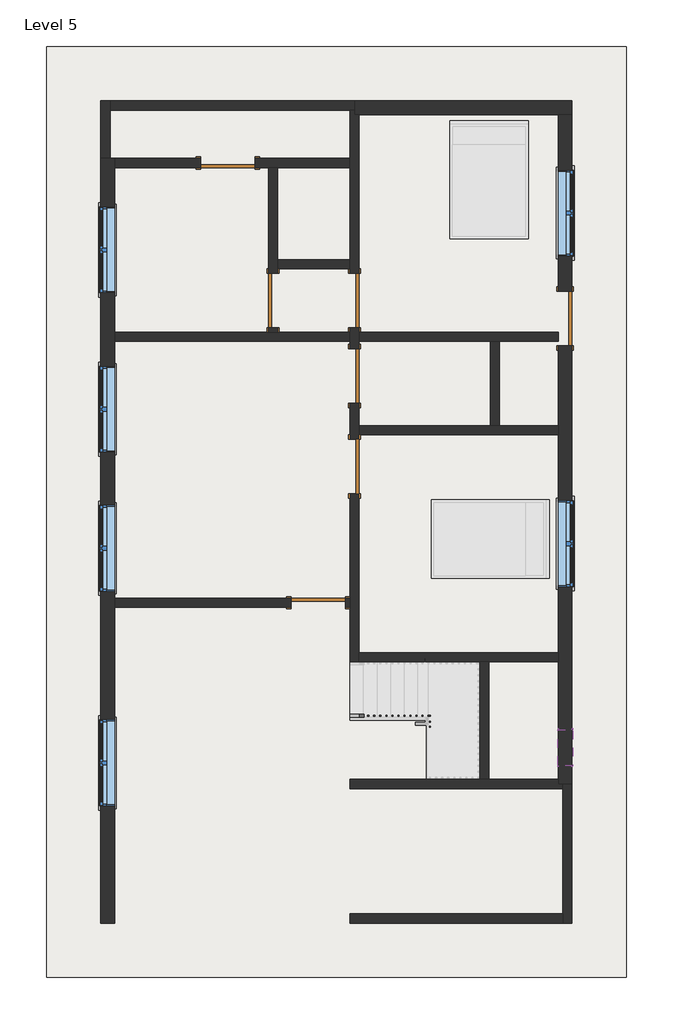
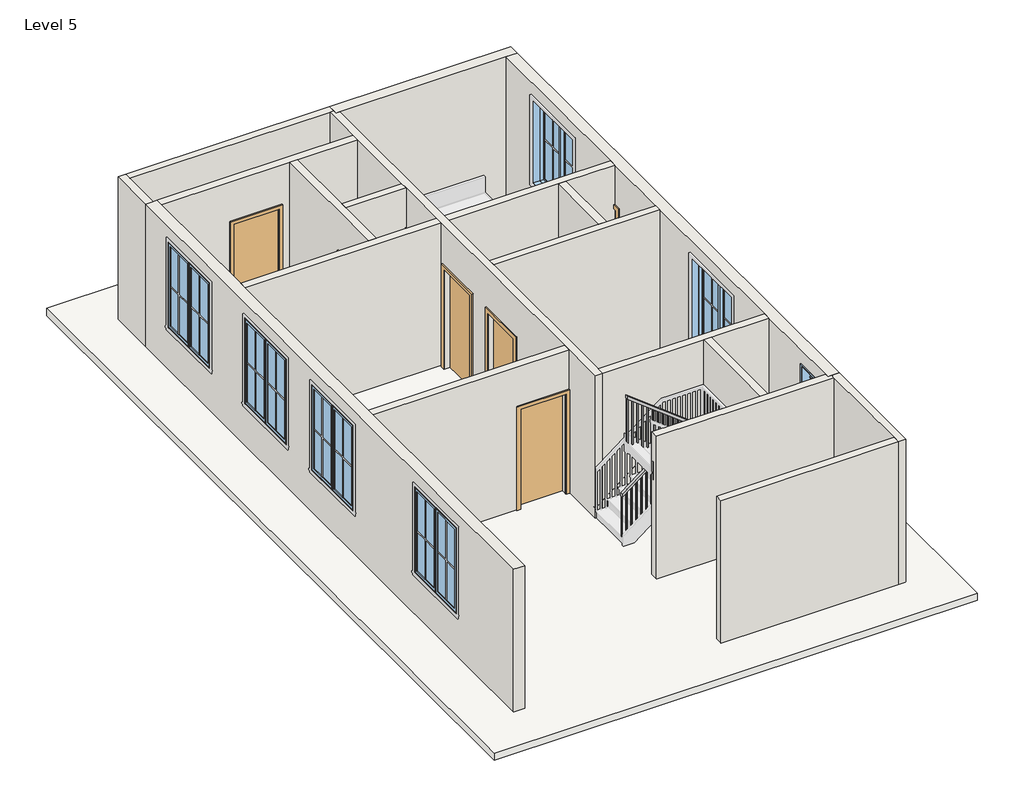
# One storey, part 1 of 2: 18 walls, 7 doors, 7 windows, 1 railing, 1 roof.
"""IFC4 building model written with IfcOpenShell, lengths in millimetres."""

from ifc_helpers import new_model, si_unit, frame, origin, place, context, project, spatial, polyline, outline, extrude, faceted_brep, transform, mapped, element, save
from components import door_686f89d2, door_16372e1c, door_0ca8825f, window_9ac97e1a, window_f2d8fef0

model = new_model("IFC4")

# Units and contexts
model_context = context("Model", 3, world=origin())
ifc_project = project(units=[si_unit("LENGTHUNIT", "METRE", prefix="MILLI")], contexts=[model_context])

# Site, building, storey
site = spatial("IfcSite", under=ifc_project)
building = spatial("IfcBuilding", under=site)
storey = spatial("IfcBuildingStorey", under=building, Name="Level 5", Elevation=9601.2)

# Doors
placement = place(None, origin())
door_shape = door_686f89d2(model_context)
element("IfcDoor", 1, ObjectType="Single-Flush : 36\" x 84\"", at=placement, inside=storey, context=model_context, shape_type="MappedRepresentation", body=[
    mapped(door_shape, transform((-2318.0415352, 3143.9226491, 9601.2), x_axis=(0.0, -1.0, 0.0), y_axis=(1.0, 0.0, 0.0), z_axis=(0.0, 0.0, 1.0))),
])
element("IfcDoor", 2, ObjectType="Single-Flush : 36\" x 84\"", at=placement, inside=storey, context=model_context, shape_type="MappedRepresentation", body=[
    mapped(door_shape, transform((-946.4415352, 3143.7222669, 9601.2), x_axis=(0.0, 1.0, 0.0), y_axis=(-1.0, 0.0, 0.0), z_axis=(0.0, 0.0, 1.0))),
])
element("IfcDoor", 3, ObjectType="Single-Flush : 36\" x 84\"", at=placement, inside=storey, context=model_context, shape_type="MappedRepresentation", body=[
    mapped(door_shape, transform((-946.4415352, 1874.1230313, 9601.2), x_axis=(0.0, 1.0, 0.0), y_axis=(-1.0, 0.0, 0.0), z_axis=(0.0, 0.0, 1.0))),
])
element("IfcDoor", 4, ObjectType="Single-Flush : 36\" x 84\"", at=placement, inside=storey, context=model_context, shape_type="MappedRepresentation", body=[
    mapped(door_shape, transform((-946.4415352, 350.1230313, 9601.2), x_axis=(0.0, 1.0, 0.0), y_axis=(-1.0, 0.0, 0.0), z_axis=(0.0, 0.0, 1.0))),
])
element("IfcDoor", 5, ObjectType="Single-Flush : 36\" x 84\"", at=placement, inside=storey, context=model_context, shape_type="MappedRepresentation", body=[
    mapped(door_shape, transform((-3080.0415352, 5453.9645078, 9601.2), x_axis=(1.0, 0.0, 0.0), y_axis=(0.0, 1.0, 0.0), z_axis=(0.0, 0.0, 1.0))),
])
door_2_shape = door_16372e1c(model_context)
element("IfcDoor", 6, ObjectType="Single-Flush : 36\" x 84\"", at=placement, inside=storey, context=model_context, shape_type="MappedRepresentation", body=[
    mapped(door_2_shape, transform((-1556.0415352, -1935.8769687, 9601.2), x_axis=(1.0, 0.0, 0.0), y_axis=(0.0, 1.0, 0.0), z_axis=(0.0, 0.0, 1.0))),
])
door_3_shape = door_0ca8825f(model_context)
element("IfcDoor", 7, ObjectType="Single-Flush : 36\" x 84\"", at=placement, inside=storey, context=model_context, shape_type="MappedRepresentation", body=[
    mapped(door_3_shape, transform((2596.8584648, 2839.3230313, 9601.2), x_axis=(0.0, -1.0, 0.0), y_axis=(1.0, 0.0, 0.0), z_axis=(0.0, 0.0, 1.0))),
])

# Railing
element("IfcRailing", 8, ObjectType="Handrail - Rectangular", at=placement, inside=storey, context=model_context, shape_type="SolidModel", body=[
    faceted_brep([(-1022.6415352, -3810.4539367, 10684.9333333), (-1022.6415352, -3810.4539367, 10620.7783974), (-1022.6415352, -3861.2539367, 10620.7783974), (-1022.6415352, -3861.2539367, 10684.9333333), (218.4221038, -3810.4539367, 11642.1605883), (269.2221038, -3810.4539367, 11617.1874824), (269.2221038, -3861.2539367, 11617.1874824), (218.4221038, -3861.2539367, 11642.1605883), (218.4221038, -3810.4539367, 11700.9333333), (269.2221038, -3810.4539367, 11650.1333333), (269.2221038, -3861.2539367, 11650.1333333), (218.4221038, -3861.2539367, 11700.9333333), (345.4221038, -3810.4539367, 11700.9333333), (345.4221038, -3810.4539367, 11650.1333333), (294.6221038, -3861.2539367, 11650.1333333), (294.6221038, -3861.2539367, 11700.9333333), (345.4221038, -3937.4539367, 11700.9333333), (345.4221038, -3937.4539367, 11650.1333333), (294.6221038, -3937.4539367, 11650.1333333), (294.6221038, -3937.4539367, 11700.9333333), (345.4221038, -3993.2769687, 11700.9333333), (294.6221038, -3993.2769687, 11700.9333333), (294.6221038, -4044.0769687, 11650.1333333), (345.4221038, -4044.0769687, 11650.1333333)], [[[0, 1, 2, 3]], [[1, 0, 4, 5]], [[2, 1, 5, 6]], [[3, 2, 6, 7]], [[0, 3, 7, 4]], [[5, 4, 8, 9]], [[6, 5, 9, 10]], [[7, 6, 10, 11]], [[4, 7, 11, 8]], [[9, 8, 12, 13]], [[10, 9, 13, 14]], [[11, 10, 14, 15]], [[8, 11, 15, 12]], [[13, 12, 16, 17]], [[14, 13, 17, 18]], [[15, 14, 18, 19]], [[12, 15, 19, 16]], [[20, 21, 22, 23]], [[17, 16, 20, 23]], [[18, 17, 23, 22]], [[19, 18, 22, 21]], [[16, 19, 21, 20]]]),
    faceted_brep([(345.4221038, -3993.2769687, 11700.9333333), (345.4221038, -4044.0769687, 11650.1333333), (294.6221038, -4044.0769687, 11650.1333333), (294.6221038, -3993.2769687, 11700.9333333), (345.4221038, -3993.2769687, 11831.0848366), (294.6221038, -3993.2769687, 11806.1117307), (294.6221038, -4044.0769687, 11806.1117307), (345.4221038, -4044.0769687, 11831.0848366)], [[[0, 1, 2, 3]], [[4, 5, 6, 7]], [[1, 0, 4, 7]], [[2, 1, 7, 6]], [[3, 2, 6, 5]], [[0, 3, 5, 4]]]),
    faceted_brep([(345.4221038, -4044.0769687, 11831.0848366), (294.6221038, -4044.0769687, 11806.1117307), (294.6221038, -3993.2769687, 11806.1117307), (345.4221038, -3993.2769687, 11831.0848366), (-1022.6415352, -4044.0769687, 12886.2666667), (-1022.6415352, -3993.2769687, 12886.2666667), (-1022.6415352, -3993.2769687, 12822.1117307), (-1022.6415352, -4044.0769687, 12822.1117307)], [[[0, 1, 2, 3]], [[4, 5, 6, 7]], [[1, 0, 4, 7]], [[2, 1, 7, 6]], [[3, 2, 6, 5]], [[0, 3, 5, 4]]]),
    extrude(outline(polyline([(12797.9018032, -991.2528962), (12812.5949894, -1010.3028962), (11802.5333333, -1010.3028962), (11802.5333333, -991.2528962), (12797.9018032, -991.2528962)])), frame((0.0, -4028.2019687, 0.0), z_axis=(0.0, 1.0, 0.0), x_axis=(0.0, 0.0, 1.0)), (0.0, 0.0, 1.0), 19.05),
    extrude(outline(polyline([(12719.5381431, -889.6528962), (12734.2313294, -908.7028962), (11802.5333333, -908.7028962), (11802.5333333, -889.6528962), (12719.5381431, -889.6528962)])), frame((0.0, -4028.2019687, 0.0), z_axis=(0.0, 1.0, 0.0), x_axis=(0.0, 0.0, 1.0)), (0.0, 0.0, 1.0), 19.05),
    extrude(outline(polyline([(12641.1744831, -788.0528962), (12655.8676694, -807.1028962), (11802.5333333, -807.1028962), (11802.5333333, -788.0528962), (12641.1744831, -788.0528962)])), frame((0.0, -4028.2019687, 0.0), z_axis=(0.0, 1.0, 0.0), x_axis=(0.0, 0.0, 1.0)), (0.0, 0.0, 1.0), 19.05),
    extrude(outline(polyline([(12562.8108231, -686.4528962), (12577.5040093, -705.5028962), (11633.2, -705.5028962), (11633.2, -686.4528962), (12562.8108231, -686.4528962)])), frame((0.0, -4028.2019687, 0.0), z_axis=(0.0, 1.0, 0.0), x_axis=(0.0, 0.0, 1.0)), (0.0, 0.0, 1.0), 19.05),
    extrude(outline(polyline([(12484.447163, -584.8528962), (12499.1403493, -603.9028962), (11633.2, -603.9028962), (11633.2, -584.8528962), (12484.447163, -584.8528962)])), frame((0.0, -4028.2019687, 0.0), z_axis=(0.0, 1.0, 0.0), x_axis=(0.0, 0.0, 1.0)), (0.0, 0.0, 1.0), 19.05),
    extrude(outline(polyline([(12406.083503, -483.2528962), (12420.7766892, -502.3028962), (11463.8666667, -502.3028962), (11463.8666667, -483.2528962), (12406.083503, -483.2528962)])), frame((0.0, -4028.2019687, 0.0), z_axis=(0.0, 1.0, 0.0), x_axis=(0.0, 0.0, 1.0)), (0.0, 0.0, 1.0), 19.05),
    extrude(outline(polyline([(12327.7198429, -381.6528962), (12342.4130292, -400.7028962), (11463.8666667, -400.7028962), (11463.8666667, -381.6528962), (12327.7198429, -381.6528962)])), frame((0.0, -4028.2019687, 0.0), z_axis=(0.0, 1.0, 0.0), x_axis=(0.0, 0.0, 1.0)), (0.0, 0.0, 1.0), 19.05),
    extrude(outline(polyline([(12249.3561829, -280.0528962), (12264.0493691, -299.1028962), (11294.5333333, -299.1028962), (11294.5333333, -280.0528962), (12249.3561829, -280.0528962)])), frame((0.0, -4028.2019687, 0.0), z_axis=(0.0, 1.0, 0.0), x_axis=(0.0, 0.0, 1.0)), (0.0, 0.0, 1.0), 19.05),
    extrude(outline(polyline([(12170.9925228, -178.4528962), (12185.6857091, -197.5028962), (11294.5333333, -197.5028962), (11294.5333333, -178.4528962), (12170.9925228, -178.4528962)])), frame((0.0, -4028.2019687, 0.0), z_axis=(0.0, 1.0, 0.0), x_axis=(0.0, 0.0, 1.0)), (0.0, 0.0, 1.0), 19.05),
    extrude(outline(polyline([(12092.6288628, -76.8528962), (12107.322049, -95.9028962), (11125.2, -95.9028962), (11125.2, -76.8528962), (12092.6288628, -76.8528962)])), frame((0.0, -4028.2019687, 0.0), z_axis=(0.0, 1.0, 0.0), x_axis=(0.0, 0.0, 1.0)), (0.0, 0.0, 1.0), 19.05),
    extrude(outline(polyline([(12014.2652027, 24.7471038), (12028.958389, 5.6971038), (11125.2, 5.6971038), (11125.2, 24.7471038), (12014.2652027, 24.7471038)])), frame((0.0, -4028.2019687, 0.0), z_axis=(0.0, 1.0, 0.0), x_axis=(0.0, 0.0, 1.0)), (0.0, 0.0, 1.0), 19.05),
    extrude(outline(polyline([(11935.9015427, 126.3471038), (11950.5947289, 107.2971038), (11125.2, 107.2971038), (11125.2, 126.3471038), (11935.9015427, 126.3471038)])), frame((0.0, -4028.2019687, 0.0), z_axis=(0.0, 1.0, 0.0), x_axis=(0.0, 0.0, 1.0)), (0.0, 0.0, 1.0), 19.05),
    extrude(outline(polyline([(11857.5378826, 227.9471038), (11872.2310689, 208.8971038), (10955.8666667, 208.8971038), (10955.8666667, 227.9471038), (11857.5378826, 227.9471038)])), frame((0.0, -4028.2019687, 0.0), z_axis=(0.0, 1.0, 0.0), x_axis=(0.0, 0.0, 1.0)), (0.0, 0.0, 1.0), 19.05),
    extrude(outline(polyline([(310.4971038, -3927.9289367), (329.5471038, -3927.9289367), (329.5471038, -3946.9789367), (310.4971038, -3946.9789367), (310.4971038, -3927.9289367)])), frame((0.0, 0.0, 10786.5333333), z_axis=(0.0, 0.0, 1.0), x_axis=(1.0, 0.0, 0.0)), (0.0, 0.0, 1.0), 863.6),
    extrude(outline(polyline([(288.6334648, -3845.3789367), (288.6334648, -3826.3289367), (307.6834648, -3826.3289367), (307.6834648, -3845.3789367), (288.6334648, -3845.3789367)])), frame((0.0, 0.0, 10786.5333333), z_axis=(0.0, 0.0, 1.0), x_axis=(1.0, 0.0, 0.0)), (0.0, 0.0, 1.0), 863.6),
    extrude(outline(polyline([(11568.4889111, 206.0834648), (11553.7957248, 187.0334648), (10617.2, 187.0334648), (10617.2, 206.0834648), (11568.4889111, 206.0834648)])), frame((0.0, -3845.3789367, 0.0), z_axis=(0.0, 1.0, 0.0), x_axis=(0.0, 0.0, 1.0)), (0.0, 0.0, 1.0), 19.05),
    extrude(outline(polyline([(11490.125251, 104.4834648), (11475.4320648, 85.4334648), (10447.8666667, 85.4334648), (10447.8666667, 104.4834648), (11490.125251, 104.4834648)])), frame((0.0, -3845.3789367, 0.0), z_axis=(0.0, 1.0, 0.0), x_axis=(0.0, 0.0, 1.0)), (0.0, 0.0, 1.0), 19.05),
    extrude(outline(polyline([(11411.761591, 2.8834648), (11397.0684047, -16.1665352), (10447.8666667, -16.1665352), (10447.8666667, 2.8834648), (11411.761591, 2.8834648)])), frame((0.0, -3845.3789367, 0.0), z_axis=(0.0, 1.0, 0.0), x_axis=(0.0, 0.0, 1.0)), (0.0, 0.0, 1.0), 19.05),
    extrude(outline(polyline([(11333.3979309, -98.7165352), (11318.7047447, -117.7665352), (10447.8666667, -117.7665352), (10447.8666667, -98.7165352), (11333.3979309, -98.7165352)])), frame((0.0, -3845.3789367, 0.0), z_axis=(0.0, 1.0, 0.0), x_axis=(0.0, 0.0, 1.0)), (0.0, 0.0, 1.0), 19.05),
    extrude(outline(polyline([(11255.0342709, -200.3165352), (11240.3410846, -219.3665352), (10278.5333333, -219.3665352), (10278.5333333, -200.3165352), (11255.0342709, -200.3165352)])), frame((0.0, -3845.3789367, 0.0), z_axis=(0.0, 1.0, 0.0), x_axis=(0.0, 0.0, 1.0)), (0.0, 0.0, 1.0), 19.05),
    extrude(outline(polyline([(11176.6706109, -301.9165352), (11161.9774246, -320.9665352), (10278.5333333, -320.9665352), (10278.5333333, -301.9165352), (11176.6706109, -301.9165352)])), frame((0.0, -3845.3789367, 0.0), z_axis=(0.0, 1.0, 0.0), x_axis=(0.0, 0.0, 1.0)), (0.0, 0.0, 1.0), 19.05),
    extrude(outline(polyline([(11098.3069508, -403.5165352), (11083.6137645, -422.5665352), (10109.2, -422.5665352), (10109.2, -403.5165352), (11098.3069508, -403.5165352)])), frame((0.0, -3845.3789367, 0.0), z_axis=(0.0, 1.0, 0.0), x_axis=(0.0, 0.0, 1.0)), (0.0, 0.0, 1.0), 19.05),
    extrude(outline(polyline([(11019.9432908, -505.1165352), (11005.2501045, -524.1665352), (10109.2, -524.1665352), (10109.2, -505.1165352), (11019.9432908, -505.1165352)])), frame((0.0, -3845.3789367, 0.0), z_axis=(0.0, 1.0, 0.0), x_axis=(0.0, 0.0, 1.0)), (0.0, 0.0, 1.0), 19.05),
    extrude(outline(polyline([(10941.5796307, -606.7165352), (10926.8864445, -625.7665352), (9939.8666667, -625.7665352), (9939.8666667, -606.7165352), (10941.5796307, -606.7165352)])), frame((0.0, -3845.3789367, 0.0), z_axis=(0.0, 1.0, 0.0), x_axis=(0.0, 0.0, 1.0)), (0.0, 0.0, 1.0), 19.05),
    extrude(outline(polyline([(10863.2159707, -708.3165352), (10848.5227844, -727.3665352), (9939.8666667, -727.3665352), (9939.8666667, -708.3165352), (10863.2159707, -708.3165352)])), frame((0.0, -3845.3789367, 0.0), z_axis=(0.0, 1.0, 0.0), x_axis=(0.0, 0.0, 1.0)), (0.0, 0.0, 1.0), 19.05),
    extrude(outline(polyline([(10784.8523106, -809.9165352), (10770.1591244, -828.9665352), (9770.5333333, -828.9665352), (9770.5333333, -809.9165352), (10784.8523106, -809.9165352)])), frame((0.0, -3845.3789367, 0.0), z_axis=(0.0, 1.0, 0.0), x_axis=(0.0, 0.0, 1.0)), (0.0, 0.0, 1.0), 19.05),
    extrude(outline(polyline([(10706.4886506, -911.5165352), (10691.7954643, -930.5665352), (9770.5333333, -930.5665352), (9770.5333333, -911.5165352), (10706.4886506, -911.5165352)])), frame((0.0, -3845.3789367, 0.0), z_axis=(0.0, 1.0, 0.0), x_axis=(0.0, 0.0, 1.0)), (0.0, 0.0, 1.0), 19.05),
    extrude(outline(polyline([(310.4971038, -4009.1519687), (329.5471038, -4009.1519687), (329.5471038, -4028.2019687), (310.4971038, -4028.2019687), (310.4971038, -4009.1519687)])), frame((0.0, 0.0, 10786.5333333), z_axis=(0.0, 0.0, 1.0), x_axis=(1.0, 0.0, 0.0)), (0.0, 0.0, 1.0), 863.6),
    extrude(outline(polyline([(310.4971038, -3845.3789367), (310.4971038, -3826.3289367), (329.5471038, -3826.3289367), (329.5471038, -3845.3789367), (310.4971038, -3845.3789367)])), frame((0.0, 0.0, 10786.5333333), z_axis=(0.0, 0.0, 1.0), x_axis=(1.0, 0.0, 0.0)), (0.0, 0.0, 1.0), 863.6),
    extrude(outline(polyline([(12807.4185445, -1003.5915352), (12822.1117307, -1022.6415352), (11802.5333333, -1022.6415352), (11802.5333333, -1003.5915352), (12807.4185445, -1003.5915352)])), frame((0.0, -4028.2019687, 0.0), z_axis=(0.0, 1.0, 0.0), x_axis=(0.0, 0.0, 1.0)), (0.0, 0.0, 1.0), 19.05),
    extrude(outline(polyline([(10635.4715837, -1003.5915352), (10620.7783974, -1022.6415352), (9770.5333333, -1022.6415352), (9770.5333333, -1003.5915352), (10635.4715837, -1003.5915352)])), frame((0.0, -3845.3789367, 0.0), z_axis=(0.0, 1.0, 0.0), x_axis=(0.0, 0.0, 1.0)), (0.0, 0.0, 1.0), 19.05),
])

# Roof
element("IfcRoof", 9, ObjectType="ROOF 6\"", at=placement, inside=storey, context=model_context, shape_type="SweptSolid", body=[
    extrude(outline(polyline([(-6128.0415352, 7411.3230313), (3625.5584648, 7411.3230313), (3625.5584648, -8235.0769687), (-6128.0415352, -8235.0769687), (-6128.0415352, 7411.3230313)])), frame((0.0, 0.0, 9448.8), z_axis=(0.0, 0.0, 1.0), x_axis=(1.0, 0.0, 0.0)), (0.0, 0.0, 1.0), 152.4),
])

# Walls
element("IfcWall", 10, ObjectType="WALL 6\"", at=placement, inside=storey, context=model_context, shape_type="Brep", body=[
    faceted_brep([(-5061.2415352, 5531.7230313, 9601.2), (-5061.2415352, 6344.5230313, 9601.2), (-5061.2415352, 6496.9230313, 9601.2), (-5061.2415352, 6496.9230313, 12649.2), (-5061.2415352, 6344.5230313, 12649.2), (-5061.2415352, 5531.7230313, 12649.2), (-5213.6415352, 5531.7230313, 9601.2), (-5213.6415352, 5531.7230313, 12649.2), (-5213.6415352, 6496.9230313, 12649.2), (-5213.6415352, 6496.9230313, 9601.2)], [[[0, 1, 2, 3, 4, 5]], [[6, 7, 8, 9]], [[2, 1, 0, 6, 9]], [[0, 5, 7, 6]], [[3, 2, 9, 8]], [[5, 4, 3, 8, 7]]]),
])
element("IfcWall", 11, ObjectType="WALL 6\"", at=placement, inside=storey, context=model_context, shape_type="Brep", body=[
    faceted_brep([(-5061.2415352, 6344.5230313, 9601.2), (-1022.6415352, 6344.5230313, 9601.2), (-946.4415352, 6344.5230313, 9601.2), (-946.4415352, 6344.5230313, 12649.2), (-1022.6415352, 6344.5230313, 12649.2), (-5061.2415352, 6344.5230313, 12649.2), (-5061.2415352, 6496.9230313, 9601.2), (-5061.2415352, 6496.9230313, 12649.2), (-946.4415352, 6496.9230313, 12649.2), (-946.4415352, 6496.9230313, 9601.2)], [[[0, 1, 2, 3, 4, 5]], [[6, 7, 8, 9]], [[2, 1, 0, 6, 9]], [[3, 2, 9, 8]], [[0, 5, 7, 6]], [[5, 4, 3, 8, 7]]]),
])
element("IfcWall", 12, ObjectType="WALL 6\"", at=placement, inside=storey, context=model_context, shape_type="Brep", body=[
    faceted_brep([(-1022.6415352, 1416.9230313, 9601.2), (-1022.6415352, 807.3230313, 9601.2), (-1022.6415352, 807.3230313, 11734.8), (-1022.6415352, -107.0769687, 11734.8), (-1022.6415352, -107.0769687, 9601.2), (-1022.6415352, -1859.6769687, 9601.2), (-1022.6415352, -2012.0769687, 9601.2), (-1022.6415352, -2926.4769687, 9601.2), (-1022.6415352, -2926.4769687, 12649.2), (-1022.6415352, -2012.0769687, 12649.2), (-1022.6415352, -1859.6769687, 12649.2), (-1022.6415352, 2458.3230313, 12649.2), (-1022.6415352, 2610.7230313, 12649.2), (-1022.6415352, 3677.1222669, 12649.2), (-1022.6415352, 3829.5222669, 12649.2), (-1022.6415352, 5377.7645078, 12649.2), (-1022.6415352, 5530.1645078, 12649.2), (-1022.6415352, 6344.5230313, 12649.2), (-1022.6415352, 6344.5230313, 9601.2), (-1022.6415352, 5530.1645078, 9601.2), (-1022.6415352, 5377.7645078, 9601.2), (-1022.6415352, 3829.5222669, 9601.2), (-1022.6415352, 3677.1222669, 9601.2), (-1022.6415352, 3600.9222669, 9601.2), (-1022.6415352, 3600.9222669, 11734.8), (-1022.6415352, 2686.5222669, 11734.8), (-1022.6415352, 2686.5222669, 9601.2), (-1022.6415352, 2610.7230313, 9601.2), (-1022.6415352, 2458.3230313, 9601.2), (-1022.6415352, 2331.3230313, 9601.2), (-1022.6415352, 2331.3230313, 11734.8), (-1022.6415352, 1416.9230313, 11734.8), (-870.2415352, 807.3230313, 11734.8), (-870.2415352, 807.3230313, 9601.2), (-870.2415352, 883.5230313, 9601.2), (-870.2415352, 1035.9230313, 9601.2), (-870.2415352, 1416.9230313, 9601.2), (-870.2415352, 1416.9230313, 11734.8), (-870.2415352, 2331.3230313, 11734.8), (-870.2415352, 2331.3230313, 9601.2), (-870.2415352, 2458.3230313, 9601.2), (-870.2415352, 2610.7230313, 9601.2), (-870.2415352, 2686.5222669, 9601.2), (-870.2415352, 2686.5222669, 11734.8), (-870.2415352, 3600.9222669, 11734.8), (-870.2415352, 3600.9222669, 9601.2), (-870.2415352, 6268.3230313, 9601.2), (-870.2415352, 6268.3230313, 12649.2), (-870.2415352, 2610.7230313, 12649.2), (-870.2415352, 2458.3230313, 12649.2), (-870.2415352, 1035.9230313, 12649.2), (-870.2415352, 883.5230313, 12649.2), (-870.2415352, -2774.0769687, 12649.2), (-870.2415352, -2926.4769687, 12649.2), (-870.2415352, -2926.4769687, 9601.2), (-870.2415352, -2774.0769687, 9601.2), (-870.2415352, -107.0769687, 9601.2), (-870.2415352, -107.0769687, 11734.8), (-946.4415352, 6344.5230313, 9601.2), (-946.4415352, 6268.3230313, 9601.2), (-946.4415352, 6344.5230313, 12649.2), (-946.4415352, 6268.3230313, 12649.2)], [[[0, 1, 2, 3, 4, 5, 6, 7, 8, 9, 10, 11, 12, 13, 14, 15, 16, 17, 18, 19, 20, 21, 22, 23, 24, 25, 26, 27, 28, 29, 30, 31]], [[32, 33, 34, 35, 36, 37, 38, 39, 40, 41, 42, 43, 44, 45, 46, 47, 48, 49, 50, 51, 52, 53, 54, 55, 56, 57]], [[46, 45, 23, 22, 21, 20, 19, 18, 58, 59]], [[42, 41, 40, 39, 29, 28, 27, 26]], [[56, 55, 54, 7, 6, 5, 4]], [[36, 35, 34, 33, 1, 0]], [[18, 17, 60, 58]], [[60, 61, 59, 58]], [[61, 47, 46, 59]], [[8, 7, 54, 53]], [[24, 23, 45, 44]], [[25, 24, 44, 43]], [[26, 25, 43, 42]], [[30, 29, 39, 38]], [[31, 30, 38, 37]], [[0, 31, 37, 36]], [[2, 1, 33, 32]], [[3, 2, 32, 57]], [[4, 3, 57, 56]], [[17, 16, 15, 14, 13, 12, 11, 10, 9, 8, 53, 52, 51, 50, 49, 48, 47, 61, 60]]]),
])
element("IfcWall", 13, ObjectType="WALL 6\"", at=placement, inside=storey, context=model_context, shape_type="Brep", body=[
    faceted_brep([(2482.5584648, -2774.0769687, 9601.2), (-870.2415352, -2774.0769687, 9601.2), (-870.2415352, -2774.0769687, 12649.2), (2482.5584648, -2774.0769687, 12649.2), (2482.5584648, -2926.4769687, 9601.2), (2482.5584648, -2926.4769687, 12649.2), (1314.1584648, -2926.4769687, 12649.2), (1161.7584648, -2926.4769687, 12649.2), (-870.2415352, -2926.4769687, 12649.2), (-870.2415352, -2926.4769687, 9601.2), (1161.7584648, -2926.4769687, 9601.2), (1314.1584648, -2926.4769687, 9601.2)], [[[0, 1, 2, 3]], [[4, 5, 6, 7, 8, 9, 10, 11]], [[1, 0, 4, 11, 10, 9]], [[2, 1, 9, 8]], [[0, 3, 5, 4]], [[3, 2, 8, 7, 6, 5]]]),
])
element("IfcWall", 14, ObjectType="WALL 6\"", at=placement, inside=storey, context=model_context, shape_type="Brep", body=[
    faceted_brep([(2558.7584648, -4983.8769687, 9601.2), (2558.7584648, -5060.0769687, 9601.2), (2558.7584648, -7168.2769687, 9601.2), (2558.7584648, -7320.6769687, 9601.2), (2558.7584648, -7320.6769687, 12649.2), (2558.7584648, -7168.2769687, 12649.2), (2558.7584648, -5060.0769687, 12649.2), (2558.7584648, -4983.8769687, 12649.2), (2711.1584648, -4983.8769687, 9601.2), (2711.1584648, -4983.8769687, 12649.2), (2711.1584648, -7320.6769687, 12649.2), (2711.1584648, -7320.6769687, 9601.2)], [[[0, 1, 2, 3, 4, 5, 6, 7]], [[8, 9, 10, 11]], [[3, 2, 1, 0, 8, 11]], [[0, 7, 9, 8]], [[4, 3, 11, 10]], [[7, 6, 5, 4, 10, 9]]]),
])
element("IfcWall", 15, ObjectType="WALL 6\"", at=placement, inside=storey, context=model_context, shape_type="SweptSolid", body=[
    extrude(outline(polyline([(-1022.6415352, -7168.2769687), (2558.7584648, -7168.2769687), (2558.7584648, -7320.6769687), (-1022.6415352, -7320.6769687), (-1022.6415352, -7168.2769687)])), frame((0.0, 0.0, 9601.2), z_axis=(0.0, 0.0, 1.0), x_axis=(1.0, 0.0, 0.0)), (0.0, 0.0, 1.0), 3048.0),
])
element("IfcWall", 16, ObjectType="WALL 6\"", at=placement, inside=storey, context=model_context, shape_type="Brep", body=[
    faceted_brep([(2482.5584648, -4907.6769687, 9601.2), (1314.1584648, -4907.6769687, 9601.2), (1161.7584648, -4907.6769687, 9601.2), (-1022.6415352, -4907.6769687, 9601.2), (-1022.6415352, -4907.6769687, 12649.2), (1161.7584648, -4907.6769687, 12649.2), (1314.1584648, -4907.6769687, 12649.2), (2482.5584648, -4907.6769687, 12649.2), (2558.7584648, -5060.0769687, 9601.2), (2558.7584648, -5060.0769687, 12649.2), (-1022.6415352, -5060.0769687, 12649.2), (-1022.6415352, -5060.0769687, 9601.2), (2482.5584648, -4983.8769687, 9601.2), (2558.7584648, -4983.8769687, 9601.2), (2482.5584648, -4983.8769687, 12649.2), (2558.7584648, -4983.8769687, 12649.2)], [[[0, 1, 2, 3, 4, 5, 6, 7]], [[8, 9, 10, 11]], [[3, 2, 1, 0, 12, 13, 8, 11]], [[4, 3, 11, 10]], [[0, 7, 14, 12]], [[14, 15, 13, 12]], [[15, 9, 8, 13]], [[7, 6, 5, 4, 10, 9, 15, 14]]]),
])
element("IfcWall", 17, ObjectType="WALL 6\"", at=placement, inside=storey, context=model_context, shape_type="SweptSolid", body=[
    extrude(outline(polyline([(1161.7584648, -4907.6769687), (1161.7584648, -2926.4769687), (1314.1584648, -2926.4769687), (1314.1584648, -4907.6769687), (1161.7584648, -4907.6769687)])), frame((0.0, 0.0, 9601.2), z_axis=(0.0, 0.0, 1.0), x_axis=(1.0, 0.0, 0.0)), (0.0, 0.0, 1.0), 3048.0),
])
element("IfcWall", 18, ObjectType="WALL 6\"", at=placement, inside=storey, context=model_context, shape_type="SweptSolid", body=[
    extrude(outline(polyline([(11734.8, -1098.8415352), (9601.2, -1098.8415352), (9601.2, -1022.6415352), (12649.2, -1022.6415352), (12649.2, -4985.0415352), (9601.2, -4985.0415352), (9601.2, -2013.2415352), (11734.8, -2013.2415352), (11734.8, -1098.8415352)])), frame((0.0, -2012.0769687, 0.0), z_axis=(0.0, 1.0, 0.0), x_axis=(0.0, 0.0, 1.0)), (0.0, 0.0, 1.0), 152.4),
])
element("IfcWall", 19, ObjectType="WALL 6\"", at=placement, inside=storey, context=model_context, shape_type="Brep", body=[
    faceted_brep([(2482.5584648, 2458.3230313, 9601.2), (2482.5584648, 2458.3230313, 12649.2), (1491.9584648, 2458.3230313, 12649.2), (1339.5584648, 2458.3230313, 12649.2), (-870.2415352, 2458.3230313, 12649.2), (-870.2415352, 2458.3230313, 9601.2), (1339.5584648, 2458.3230313, 9601.2), (1491.9584648, 2458.3230313, 9601.2), (2482.5584648, 2610.7230313, 12649.2), (2482.5584648, 2610.7230313, 9601.2), (-870.2415352, 2610.7230313, 9601.2), (-870.2415352, 2610.7230313, 12649.2)], [[[0, 1, 2, 3, 4, 5, 6, 7]], [[8, 9, 10, 11]], [[9, 0, 7, 6, 5, 10]], [[1, 0, 9, 8]], [[5, 4, 11, 10]], [[1, 8, 11, 4, 3, 2]]]),
    faceted_brep([(-4985.0415352, 2458.3230313, 12649.2), (-4985.0415352, 2458.3230313, 9601.2), (-1022.6415352, 2458.3230313, 9601.2), (-1022.6415352, 2458.3230313, 12649.2), (-4985.0415352, 2610.7230313, 9601.2), (-4985.0415352, 2610.7230313, 12649.2), (-2394.2415352, 2610.7230313, 12649.2), (-2241.8415352, 2610.7230313, 12649.2), (-1022.6415352, 2610.7230313, 12649.2), (-1022.6415352, 2610.7230313, 9601.2), (-2241.8415352, 2610.7230313, 9601.2), (-2394.2415352, 2610.7230313, 9601.2)], [[[0, 1, 2, 3]], [[4, 5, 6, 7, 8, 9, 10, 11]], [[1, 4, 11, 10, 9, 2]], [[1, 0, 5, 4]], [[3, 2, 9, 8]], [[5, 0, 3, 8, 7, 6]]]),
])
element("IfcWall", 20, ObjectType="WALL 6\"", at=placement, inside=storey, context=model_context, shape_type="Brep", body=[
    faceted_brep([(-2622.8415352, 5377.7645078, 11734.8), (-2622.8415352, 5377.7645078, 9601.2), (-2394.2415352, 5377.7645078, 9601.2), (-2241.8415352, 5377.7645078, 9601.2), (-1022.6415352, 5377.7645078, 9601.2), (-1022.6415352, 5377.7645078, 12649.2), (-2241.8415352, 5377.7645078, 12649.2), (-2394.2415352, 5377.7645078, 12649.2), (-4985.0415352, 5377.7645078, 12649.2), (-4985.0415352, 5377.7645078, 9601.2), (-3537.2415352, 5377.7645078, 9601.2), (-3537.2415352, 5377.7645078, 11734.8), (-1022.6415352, 5530.1645078, 9601.2), (-2622.8415352, 5530.1645078, 9601.2), (-2622.8415352, 5530.1645078, 11734.8), (-3537.2415352, 5530.1645078, 11734.8), (-3537.2415352, 5530.1645078, 9601.2), (-4985.0415352, 5530.1645078, 9601.2), (-4985.0415352, 5530.1645078, 12649.2), (-1022.6415352, 5530.1645078, 12649.2)], [[[0, 1, 2, 3, 4, 5, 6, 7, 8, 9, 10, 11]], [[12, 13, 14, 15, 16, 17, 18, 19]], [[10, 9, 17, 16]], [[4, 3, 2, 1, 13, 12]], [[9, 8, 18, 17]], [[5, 4, 12, 19]], [[14, 13, 1, 0]], [[15, 14, 0, 11]], [[16, 15, 11, 10]], [[8, 7, 6, 5, 19, 18]]]),
])
element("IfcWall", 21, ObjectType="WALL 6\"", at=placement, inside=storey, context=model_context, shape_type="Brep", body=[
    faceted_brep([(-2394.2415352, 2686.7226491, 11734.8), (-2394.2415352, 2686.7226491, 9601.2), (-2394.2415352, 2610.7230313, 9601.2), (-2394.2415352, 2610.7230313, 12649.2), (-2394.2415352, 5377.7645078, 12649.2), (-2394.2415352, 5377.7645078, 9601.2), (-2394.2415352, 3601.1226491, 9601.2), (-2394.2415352, 3601.1226491, 11734.8), (-2241.8415352, 2610.7230313, 9601.2), (-2241.8415352, 2686.7226491, 9601.2), (-2241.8415352, 2686.7226491, 11734.8), (-2241.8415352, 3601.1226491, 11734.8), (-2241.8415352, 3601.1226491, 9601.2), (-2241.8415352, 3677.1222669, 9601.2), (-2241.8415352, 3829.5222669, 9601.2), (-2241.8415352, 5377.7645078, 9601.2), (-2241.8415352, 5377.7645078, 12649.2), (-2241.8415352, 3829.5222669, 12649.2), (-2241.8415352, 3677.1222669, 12649.2), (-2241.8415352, 2610.7230313, 12649.2)], [[[0, 1, 2, 3, 4, 5, 6, 7]], [[8, 9, 10, 11, 12, 13, 14, 15, 16, 17, 18, 19]], [[6, 5, 15, 14, 13, 12]], [[2, 1, 9, 8]], [[3, 2, 8, 19]], [[5, 4, 16, 15]], [[10, 9, 1, 0]], [[11, 10, 0, 7]], [[12, 11, 7, 6]], [[4, 3, 19, 18, 17, 16]]]),
])
element("IfcWall", 22, ObjectType="WALL 6\"", at=placement, inside=storey, context=model_context, shape_type="SweptSolid", body=[
    extrude(outline(polyline([(-1022.6415352, 3677.1222669), (-2241.8415352, 3677.1222669), (-2241.8415352, 3829.5222669), (-1022.6415352, 3829.5222669), (-1022.6415352, 3677.1222669)])), frame((0.0, 0.0, 9601.2), z_axis=(0.0, 0.0, 1.0), x_axis=(1.0, 0.0, 0.0)), (0.0, 0.0, 1.0), 3048.0),
])
element("IfcWall", 23, ObjectType="WALL 6\"", at=placement, inside=storey, context=model_context, shape_type="Brep", body=[
    faceted_brep([(-870.2415352, 883.5230313, 9601.2), (2482.5584648, 883.5230313, 9601.2), (2482.5584648, 883.5230313, 12649.2), (-870.2415352, 883.5230313, 12649.2), (-870.2415352, 1035.9230313, 9601.2), (-870.2415352, 1035.9230313, 12649.2), (1339.5584648, 1035.9230313, 12649.2), (1491.9584648, 1035.9230313, 12649.2), (2482.5584648, 1035.9230313, 12649.2), (2482.5584648, 1035.9230313, 9601.2), (1491.9584648, 1035.9230313, 9601.2), (1339.5584648, 1035.9230313, 9601.2)], [[[0, 1, 2, 3]], [[4, 5, 6, 7, 8, 9, 10, 11]], [[1, 0, 4, 11, 10, 9]], [[2, 1, 9, 8]], [[0, 3, 5, 4]], [[3, 2, 8, 7, 6, 5]]]),
])
element("IfcWall", 24, ObjectType="WALL 6\"", at=placement, inside=storey, context=model_context, shape_type="SweptSolid", body=[
    extrude(outline(polyline([(1339.5584648, 1035.9230313), (1339.5584648, 2458.3230313), (1491.9584648, 2458.3230313), (1491.9584648, 1035.9230313), (1339.5584648, 1035.9230313)])), frame((0.0, 0.0, 9601.2), z_axis=(0.0, 0.0, 1.0), x_axis=(1.0, 0.0, 0.0)), (0.0, 0.0, 1.0), 3048.0),
])
element("IfcWall", 25, ObjectType="WALL 9\"", at=placement, inside=storey, context=model_context, shape_type="Brep", body=[
    faceted_brep([(-946.4415352, 6268.3230313, 9601.2), (-870.2415352, 6268.3230313, 9601.2), (2482.5584648, 6268.3230313, 9601.2), (2711.1584648, 6268.3230313, 9601.2), (2711.1584648, 6268.3230313, 12649.2), (2482.5584648, 6268.3230313, 12649.2), (-870.2415352, 6268.3230313, 12649.2), (-946.4415352, 6268.3230313, 12649.2), (-946.4415352, 6496.9230313, 9601.2), (-946.4415352, 6496.9230313, 12649.2), (2711.1584648, 6496.9230313, 12649.2), (2711.1584648, 6496.9230313, 9601.2), (-946.4415352, 6344.5230313, 9601.2), (-946.4415352, 6344.5230313, 12649.2)], [[[0, 1, 2, 3, 4, 5, 6, 7]], [[8, 9, 10, 11]], [[3, 2, 1, 0, 12, 8, 11]], [[0, 7, 13, 9, 8, 12]], [[4, 3, 11, 10]], [[7, 6, 5, 4, 10, 9, 13]]]),
])
element("IfcWall", 26, ObjectType="WALL 9\"", at=placement, inside=storey, context=model_context, shape_type="Brep", body=[
    faceted_brep([(2482.5584648, 2382.1230313, 11734.8), (2482.5584648, 2382.1230313, 9601.2), (2482.5584648, 1035.9230313, 9601.2), (2482.5584648, 883.5230313, 9601.2), (2482.5584648, -2774.0769687, 9601.2), (2482.5584648, -2926.4769687, 9601.2), (2482.5584648, -4907.6769687, 9601.2), (2482.5584648, -4983.8769687, 9601.2), (2482.5584648, -4983.8769687, 12649.2), (2482.5584648, -4907.6769687, 12649.2), (2482.5584648, -2926.4769687, 12649.2), (2482.5584648, -2774.0769687, 12649.2), (2482.5584648, 883.5230313, 12649.2), (2482.5584648, 1035.9230313, 12649.2), (2482.5584648, 2458.3230313, 12649.2), (2482.5584648, 2610.7230313, 12649.2), (2482.5584648, 6268.3230313, 12649.2), (2482.5584648, 6268.3230313, 9601.2), (2482.5584648, 3296.5230313, 9601.2), (2482.5584648, 3296.5230313, 11734.8), (2482.5584648, 3887.0730313, 12344.4), (2482.5584648, 3887.0730313, 10515.6), (2482.5584648, 5334.8730313, 10515.6), (2482.5584648, 5334.8730313, 12344.4), (2482.5584648, -1669.1769687, 12344.4), (2482.5584648, -1669.1769687, 10515.6), (2482.5584648, -221.3769687, 10515.6), (2482.5584648, -221.3769687, 12344.4), (2482.5584648, -4069.4769687, 12344.4), (2482.5584648, -4679.0769687, 12344.4), (2482.5584648, -4679.0769687, 11734.8), (2482.5584648, -4069.4769687, 11734.8), (2711.1584648, -4983.8769687, 9601.2), (2711.1584648, 2382.1230313, 9601.2), (2711.1584648, 2382.1230313, 11734.8), (2711.1584648, 3296.5230313, 11734.8), (2711.1584648, 3296.5230313, 9601.2), (2711.1584648, 6268.3230313, 9601.2), (2711.1584648, 6268.3230313, 12649.2), (2711.1584648, -4983.8769687, 12649.2), (2711.1584648, 3887.0730313, 12344.4), (2711.1584648, 5334.8730313, 12344.4), (2711.1584648, 5334.8730313, 10515.6), (2711.1584648, 3887.0730313, 10515.6), (2711.1584648, -1669.1769687, 12344.4), (2711.1584648, -221.3769687, 12344.4), (2711.1584648, -221.3769687, 10515.6), (2711.1584648, -1669.1769687, 10515.6), (2711.1584648, -4069.4769687, 12344.4), (2711.1584648, -4069.4769687, 11734.8), (2711.1584648, -4679.0769687, 11734.8), (2711.1584648, -4679.0769687, 12344.4), (2558.7584648, -4983.8769687, 9601.2), (2558.7584648, -4983.8769687, 12649.2)], [[[0, 1, 2, 3, 4, 5, 6, 7, 8, 9, 10, 11, 12, 13, 14, 15, 16, 17, 18, 19], [20, 21, 22, 23], [24, 25, 26, 27], [28, 29, 30, 31]], [[32, 33, 34, 35, 36, 37, 38, 39], [40, 41, 42, 43], [44, 45, 46, 47], [48, 49, 50, 51]], [[18, 17, 37, 36]], [[7, 6, 5, 4, 3, 2, 1, 33, 32, 52]], [[8, 7, 52, 32, 39, 53]], [[17, 16, 38, 37]], [[34, 33, 1, 0]], [[35, 34, 0, 19]], [[36, 35, 19, 18]], [[21, 20, 40, 43]], [[22, 21, 43, 42]], [[23, 22, 42, 41]], [[20, 23, 41, 40]], [[25, 24, 44, 47]], [[26, 25, 47, 46]], [[27, 26, 46, 45]], [[24, 27, 45, 44]], [[49, 48, 28, 31]], [[50, 49, 31, 30]], [[51, 50, 30, 29]], [[48, 51, 29, 28]], [[16, 15, 14, 13, 12, 11, 10, 9, 8, 53, 39, 38]]]),
])
element("IfcWall", 27, ObjectType="WALL 9\"", at=placement, inside=storey, context=model_context, shape_type="Brep", body=[
    faceted_brep([(-4985.0415352, -7320.6769687, 9601.2), (-4985.0415352, -2012.0769687, 9601.2), (-4985.0415352, -1859.6769687, 9601.2), (-4985.0415352, 2458.3230313, 9601.2), (-4985.0415352, 2610.7230313, 9601.2), (-4985.0415352, 5377.7645078, 9601.2), (-4985.0415352, 5530.1645078, 9601.2), (-4985.0415352, 5531.7230313, 9601.2), (-4985.0415352, 5531.7230313, 12649.2), (-4985.0415352, 5530.1645078, 12649.2), (-4985.0415352, 5377.7645078, 12649.2), (-4985.0415352, 2610.7230313, 12649.2), (-4985.0415352, 2458.3230313, 12649.2), (-4985.0415352, -1859.6769687, 12649.2), (-4985.0415352, -2012.0769687, 12649.2), (-4985.0415352, -7320.6769687, 12649.2), (-4985.0415352, 4718.1437696, 12344.4), (-4985.0415352, 4718.1437696, 10515.6), (-4985.0415352, 3270.3437696, 10515.6), (-4985.0415352, 3270.3437696, 12344.4), (-4985.0415352, 2039.2230313, 12344.4), (-4985.0415352, 2039.2230313, 10515.6), (-4985.0415352, 591.4230313, 10515.6), (-4985.0415352, 591.4230313, 12344.4), (-4985.0415352, -297.5769687, 12344.4), (-4985.0415352, -297.5769687, 10515.6), (-4985.0415352, -1745.3769687, 10515.6), (-4985.0415352, -1745.3769687, 12344.4), (-4985.0415352, -3904.3769687, 12344.4), (-4985.0415352, -3904.3769687, 10515.6), (-4985.0415352, -5352.1769687, 10515.6), (-4985.0415352, -5352.1769687, 12344.4), (-5213.6415352, -7320.6769687, 9601.2), (-5213.6415352, -7320.6769687, 12649.2), (-5213.6415352, 5531.7230313, 12649.2), (-5213.6415352, 5531.7230313, 9601.2), (-5213.6415352, 4718.1437696, 12344.4), (-5213.6415352, 3270.3437696, 12344.4), (-5213.6415352, 3270.3437696, 10515.6), (-5213.6415352, 4718.1437696, 10515.6), (-5213.6415352, 2039.2230313, 12344.4), (-5213.6415352, 591.4230313, 12344.4), (-5213.6415352, 591.4230313, 10515.6), (-5213.6415352, 2039.2230313, 10515.6), (-5213.6415352, -297.5769687, 12344.4), (-5213.6415352, -1745.3769687, 12344.4), (-5213.6415352, -1745.3769687, 10515.6), (-5213.6415352, -297.5769687, 10515.6), (-5213.6415352, -3904.3769687, 12344.4), (-5213.6415352, -5352.1769687, 12344.4), (-5213.6415352, -5352.1769687, 10515.6), (-5213.6415352, -3904.3769687, 10515.6), (-5061.2415352, 5531.7230313, 9601.2), (-5061.2415352, 5531.7230313, 12649.2)], [[[0, 1, 2, 3, 4, 5, 6, 7, 8, 9, 10, 11, 12, 13, 14, 15], [16, 17, 18, 19], [20, 21, 22, 23], [24, 25, 26, 27], [28, 29, 30, 31]], [[32, 33, 34, 35], [36, 37, 38, 39], [40, 41, 42, 43], [44, 45, 46, 47], [48, 49, 50, 51]], [[7, 6, 5, 4, 3, 2, 1, 0, 32, 35, 52]], [[8, 7, 52, 35, 34, 53]], [[0, 15, 33, 32]], [[17, 16, 36, 39]], [[18, 17, 39, 38]], [[19, 18, 38, 37]], [[16, 19, 37, 36]], [[21, 20, 40, 43]], [[22, 21, 43, 42]], [[23, 22, 42, 41]], [[20, 23, 41, 40]], [[25, 24, 44, 47]], [[26, 25, 47, 46]], [[27, 26, 46, 45]], [[24, 27, 45, 44]], [[29, 28, 48, 51]], [[30, 29, 51, 50]], [[31, 30, 50, 49]], [[28, 31, 49, 48]], [[15, 14, 13, 12, 11, 10, 9, 8, 53, 34, 33]]]),
])

# Windows
window_shape = window_9ac97e1a(model_context)
element("IfcWindow", 28, ObjectType="Window-Casement-Double : 57\" x 72\"", at=placement, inside=storey, context=model_context, shape_type="MappedRepresentation", body=[
    mapped(window_shape, transform((-5099.3415352, 3994.2437696, 9601.2), x_axis=(0.0, 1.0, 0.0), y_axis=(-1.0, 0.0, 0.0), z_axis=(0.0, 0.0, 1.0))),
])
element("IfcWindow", 29, ObjectType="Window-Casement-Double : 57\" x 72\"", at=placement, inside=storey, context=model_context, shape_type="MappedRepresentation", body=[
    mapped(window_shape, transform((2596.8584648, 4610.9730313, 9601.2), x_axis=(0.0, -1.0, 0.0), y_axis=(1.0, 0.0, 0.0), z_axis=(0.0, 0.0, 1.0))),
])
element("IfcWindow", 30, ObjectType="Window-Casement-Double : 57\" x 72\"", at=placement, inside=storey, context=model_context, shape_type="MappedRepresentation", body=[
    mapped(window_shape, transform((2596.8584648, -945.2769687, 9601.2), x_axis=(0.0, -1.0, 0.0), y_axis=(1.0, 0.0, 0.0), z_axis=(0.0, 0.0, 1.0))),
])
element("IfcWindow", 31, ObjectType="Window-Casement-Double : 57\" x 72\"", at=placement, inside=storey, context=model_context, shape_type="MappedRepresentation", body=[
    mapped(window_shape, transform((-5099.3415352, 1315.3230313, 9601.2), x_axis=(0.0, 1.0, 0.0), y_axis=(-1.0, 0.0, 0.0), z_axis=(0.0, 0.0, 1.0))),
])
element("IfcWindow", 32, ObjectType="Window-Casement-Double : 57\" x 72\"", at=placement, inside=storey, context=model_context, shape_type="MappedRepresentation", body=[
    mapped(window_shape, transform((-5099.3415352, -1021.4769687, 9601.2), x_axis=(0.0, 1.0, 0.0), y_axis=(-1.0, 0.0, 0.0), z_axis=(0.0, 0.0, 1.0))),
])
element("IfcWindow", 33, ObjectType="Window-Casement-Double : 57\" x 72\"", at=placement, inside=storey, context=model_context, shape_type="MappedRepresentation", body=[
    mapped(window_shape, transform((-5099.3415352, -4628.2769687, 9601.2), x_axis=(0.0, 1.0, 0.0), y_axis=(-1.0, 0.0, 0.0), z_axis=(0.0, 0.0, 1.0))),
])
window_2_shape = window_f2d8fef0(model_context)
element("IfcWindow", 34, ObjectType="Window-Louvers : 24\" x 24\"", at=placement, inside=storey, context=model_context, shape_type="MappedRepresentation", body=[
    mapped(window_2_shape, transform((2603.2084648, -4374.2769687, 10820.4), x_axis=(0.0, -1.0, 0.0), y_axis=(1.0, 0.0, 0.0), z_axis=(0.0, 0.0, 1.0))),
])

save(model, "model.ifc")

# Revit data of these elements
# Type "Single-Flush : 36\" x 84\""
#   Type Mark = "1"
#   Construction Type Id = "MDOOR"
#   Assembly Code = "C1020"
#   Analytic Construction = "Metal"
#   Thickness = 0' - 2"
#   Heat Transfer Coefficient (U) = 0.651978 BTU/(h·ft²·°F)
#   Height = 7' - 0"
#   Trim Projection Ext = 0' - 1"
#   Trim Projection Int = 0' - 1"
#   Trim Width = 0' - 3"
#   Width = 3' - 0"
#   Define Thermal Properties by = 1
#   Define Thermal Properties by = 1
#   Door Material = Door - Panel
#   Frame Material = Door - Frame
#   Visual Light Transmittance = 0
#   Solar Heat Gain Coefficient = 0
#   Function = (empty or 0)
#   Wall Closure = (empty or 0)
# Type "Handrail - Rectangular"
#   Assembly Code = "C2010400"
#   built-in parameter 1008612 = 0.0416667 (stored number, unit not read)
#   built-in parameter 1008611 = 0.0416667 (stored number, unit not read)
#   built-in parameter 1008609 = 0.333333 (stored number, unit not read)
#   built-in parameter 1008604 = 0.166667 (stored number, unit not read)
#   built-in parameter 1008603 = 0.166667 (stored number, unit not read)
#   Railing Height = 3' - 0"
#   built-in parameter 1008630 = 2
#   built-in parameter 1008610 = 2
#   built-in parameter 1008618 = Baluster - Square : 3/4"
# Type "ROOF 6\""
#   Assembly Code = "B1020"
#   Layers, outside or top first: 0' - 6" no material (function 1)
# Type "WALL 6\""
#   Assembly Code = "B2010"
#   Layers, outside or top first: 0' - 6" no material (function 1)
# Type "WALL 9\""
#   Assembly Code = "B2010"
#   Layers, outside or top first: 0' - 9" no material (function 1)
# Type "Window-Casement-Double : 57\" x 72\""
#   Type Mark = "17"
#   Fire Rating = "0.5h"
#   Assembly Code = "B2020100"
#   Analytic Construction = "Double glazing - domestic"
#   Frame Extension [instance default] = 0' - 0 1/4"
#   Window Inset [instance default] = 0' - 0"
#   Wall Thickness [instance default] = 0' - 6"
#   Interior Wall Closure [instance default] = 0' - 2 1/4"
#   Half Width = 2' - 4 1/2"
#   Visual Light Transmittance = 0.81
#   Thermal Resistance (R) = 1.8146 (h·ft²·°F)/BTU
#   Solar Heat Gain Coefficient = 0.76
#   Rough Width = 4' - 9 1/2"
#   Rough Height = 6' - 0 1/2"
#   Height = 6' - 0"
#   Heat Transfer Coefficient (U) = 0.5511 BTU/(h·ft²·°F)
#   Exterior Wall Closure [instance default] = 0' - 1 1/4"
#   Extension Jamb [instance default] = 0' - 2 1/4"
#   Default Sill Height = 3' - 0"
#   Width = 4' - 9"
#   Define Thermal Properties by = 0
#   Muntin Visibility = yes
#   Interior Trim Visibility [instance default] = yes
#   Exterior Trim Visibility [instance default] = yes
#   Extension Jamb Visibility [instance default] = yes
#   Interior Trim Material = Wood - Stained
#   Muntin Pattern = Muntin Pattern_2x2 : Muntin Pattern_2x2
#   Interior Trim = Trim-Window-Interior-Flat : Picture Frame
#   Interior Frame Material = Wood - Stained
#   Glass Panel Material = Glass
#   Exterior Trim Material = Clad - White
#   Exterior Trim = Trim-Window-Exterior-Flat : with Sill
#   Exterior Frame Material = Clad - White
#   Wall Closure = (empty or 0)
# Type "Window-Louvers : 24\" x 24\""
#   Type Mark = "18"
#   Construction Type Id = "GSP4R"
#   Assembly Code = "B20"
#   Analytic Construction = "1/8 in Pilkington single glazing"
#   Visual Light Transmittance = 0.9
#   Thermal Resistance (R) = 1.53941 (h·ft²·°F)/BTU
#   Solar Heat Gain Coefficient = 0.78
#   Max Height = 1' - 11.74264"
#   Height = 2' - 0"
#   Heat Transfer Coefficient (U) = 0.6496 BTU/(h·ft²·°F)
#   Blade Width [instance default] = 1' - 10 1/2"
#   Blade Vertical Thickness = 0' - 0.35355"
#   Blade Thickness = 0' - 0 1/4"
#   Blade Spacing = 0' - 1 1/2"
#   Blade Height = 0' - 1.85355"
#   Blade Depth = 0' - 3"
#   Blade Angle = 45.00°
#   Default Sill Height = 3' - 0"
#   Trim Projection_Exterior = 0' - 0 1/2"
#   Trim Projection_Interior = 0' - 0 1/2"
#   Trim Width_Exterior = 0' - 1 1/2"
#   Trim Width_Interior = 0' - 1 1/2"
#   Width = 2' - 0"
#   Max Blade Count = 12
#   Define Thermal Properties by = 1
#   Blade Count = 12
#   Frame Material = Birch
#   Louver Material = Birch
#   Trim Exterior Material = Birch
#   Trim Interior Material = Birch
#   Wall Closure = (empty or 0)
# Elements 1, 2, 3, 4, 5, 6, 7 (IfcDoor, "Single-Flush : 36\" x 84\"")
#   Phase Created = New Construction
#   Materials on its faces: "Door - Frame", "Door - Panel"
# Element 8 (IfcRailing, "Handrail - Rectangular")
#   Phase Created = New Construction
# Element 9 (IfcRoof, "ROOF 6\"")
#   built-in parameter 1001705 = 31.5 (stored number, unit not read)
#   built-in parameter 1001701 = -0.5 (stored number, unit not read)
#   built-in parameter 1001710 = 33615
#   Phase Created = New Construction
#   Materials on its faces: "Default Roof", "Door - Panel"
# Elements 10, 11, 14, 15, 16, 18 (IfcWall, "WALL 6\"")
#   Top Offset = 0' - 0"
#   Base Offset = 0' - 0"
#   Unconnected Height = 10' - 0"
#   wall height = 10' - 0"
#   Phase Created = New Construction
#   Base Constraint = Level 5
#   Materials on its faces: "Default Wall", "Copper"
# Elements 12, 13, 17, 19, 20, 21, 22, 23, 24 (IfcWall, "WALL 6\"")
#   Top Offset = 0' - 0"
#   Base Offset = 0' - 0"
#   Unconnected Height = 10' - 0"
#   wall height = 10' - 0"
#   Phase Created = New Construction
#   Base Constraint = Level 5
#   Materials on its faces: "Default Wall"
# Elements 25, 26, 27 (IfcWall, "WALL 9\"")
#   Top Offset = 0' - 0"
#   Base Offset = 0' - 0"
#   Unconnected Height = 10' - 0"
#   wall height = 10' - 0"
#   Phase Created = New Construction
#   Base Constraint = Level 5
#   Materials on its faces: "Default Wall", "Copper"
# Element 28 (IfcWindow, "Window-Casement-Double : 57\" x 72\"")
#   Mark = "22"
#   Window Inset = 0' - 0"
#   Interior Wall Closure = 0' - 2 1/4"
#   Frame Extension = 0' - 0 1/4"
#   Exterior Wall Closure = 0' - 1 1/4"
#   Interior Trim Visibility = yes
#   Exterior Trim Visibility = yes
#   Phase Created = New Construction
#   Materials on its faces: "Wood - Stained", "Glass", "Clad - White"
# Element 29 (IfcWindow, "Window-Casement-Double : 57\" x 72\"")
#   Mark = "23"
#   Window Inset = 0' - 0"
#   Interior Wall Closure = 0' - 2 1/4"
#   Frame Extension = 0' - 0 1/4"
#   Exterior Wall Closure = 0' - 1 1/4"
#   Interior Trim Visibility = yes
#   Exterior Trim Visibility = yes
#   Phase Created = New Construction
#   Materials on its faces: "Wood - Stained", "Glass", "Clad - White"
# Element 30 (IfcWindow, "Window-Casement-Double : 57\" x 72\"")
#   Mark = "24"
#   Window Inset = 0' - 0"
#   Interior Wall Closure = 0' - 2 1/4"
#   Frame Extension = 0' - 0 1/4"
#   Exterior Wall Closure = 0' - 1 1/4"
#   Interior Trim Visibility = yes
#   Exterior Trim Visibility = yes
#   Phase Created = New Construction
#   Materials on its faces: "Wood - Stained", "Glass", "Clad - White"
# Element 31 (IfcWindow, "Window-Casement-Double : 57\" x 72\"")
#   Mark = "25"
#   Window Inset = 0' - 0"
#   Interior Wall Closure = 0' - 2 1/4"
#   Frame Extension = 0' - 0 1/4"
#   Exterior Wall Closure = 0' - 1 1/4"
#   Interior Trim Visibility = yes
#   Exterior Trim Visibility = yes
#   Phase Created = New Construction
#   Materials on its faces: "Wood - Stained", "Glass", "Clad - White"
# Element 32 (IfcWindow, "Window-Casement-Double : 57\" x 72\"")
#   Mark = "26"
#   Window Inset = 0' - 0"
#   Interior Wall Closure = 0' - 2 1/4"
#   Frame Extension = 0' - 0 1/4"
#   Exterior Wall Closure = 0' - 1 1/4"
#   Interior Trim Visibility = yes
#   Exterior Trim Visibility = yes
#   Phase Created = New Construction
#   Materials on its faces: "Wood - Stained", "Glass", "Clad - White"
# Element 33 (IfcWindow, "Window-Casement-Double : 57\" x 72\"")
#   Mark = "27"
#   Window Inset = 0' - 0"
#   Interior Wall Closure = 0' - 2 1/4"
#   Frame Extension = 0' - 0 1/4"
#   Exterior Wall Closure = 0' - 1 1/4"
#   Interior Trim Visibility = yes
#   Exterior Trim Visibility = yes
#   Phase Created = New Construction
#   Materials on its faces: "Wood - Stained", "Glass", "Clad - White"
# Element 34 (IfcWindow, "Window-Louvers : 24\" x 24\"")
#   Mark = "28"
#   Blade Width = 1' - 10 1/2"
#   Phase Created = New Construction
#   Materials on its faces: "Birch"
# Materials
#   "Door - Panel": class "Wood", colour RGB 210 159 95, transparency 0, Cost = 0
#   "Door - Frame": colour RGB 118 70 51, transparency 0, Cost = 0
#   "Wood - Stained": class "Wood", colour RGB 224 178 126, transparency 0, Cost = 0
#   "Glass": class "Glass", colour RGB 0 128 192, transparency 0.75, Description = "Soda Lime Glass", Cost = 0
#   "Clad - White": class "Wood", colour RGB 242 242 238, transparency 0, Cost = 0
#   "Birch": class "Wood", colour RGB 224 178 126, transparency 0, Description = "Betula Alleghaniensis", Cost = 0
#   "Default Roof": colour RGB 88 101 114, transparency 0, Cost = 0
#   "Default Wall": colour RGB 128 128 128, transparency 0, Cost = 0
#   "Copper": class "Metal", colour RGB 0 0 0, transparency 0, Description = "Copper, matte finish", Cost = 0
